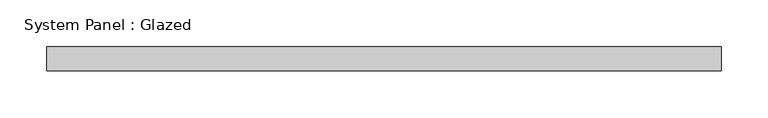
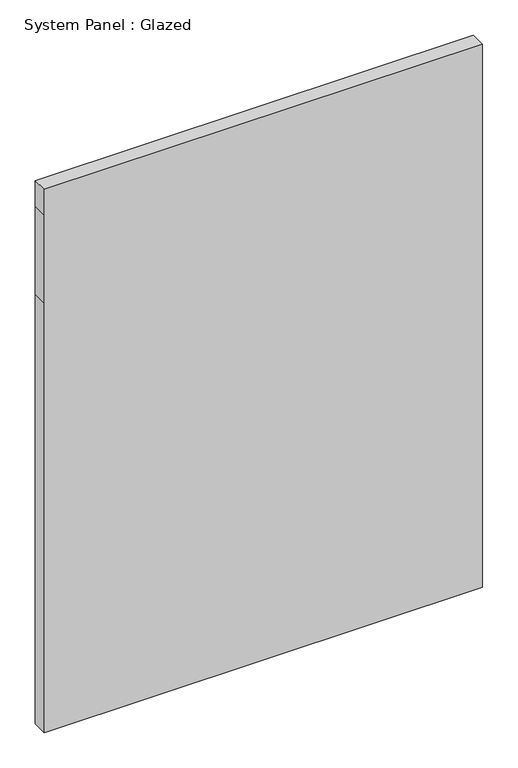
"""IFC4 building model written with IfcOpenShell, lengths in millimetres: plate geometry, System Panel : Glazed."""

from ifc_helpers import new_model, si_unit, frame, origin, place, context, project, spatial, polyline, outline, extrude, source, transform, mapped, element, save


def system_panel_glazed_be4ca357(model_context):
    return source(origin(), model_context, "Body", "SweptSolid", [
        extrude(outline(polyline([(0.0, -358.775), (0.0, 358.775), (742.6882113, 358.775), (895.0882113, 358.775), (939.5382113, 358.775), (939.5382113, -358.775), (895.0882113, -358.775), (742.6882113, -358.775), (0.0, -358.775)])), frame((0.0, 19.05, 0.0), z_axis=(0.0, 1.0, 0.0), x_axis=(0.0, 0.0, 1.0)), (0.0, 0.0, 1.0), 25.4),
    ])


if __name__ == "__main__":
    model = new_model("IFC4")
    model_context = context("Model", 3, world=origin())
    ifc_project = project(units=[si_unit("LENGTHUNIT", "METRE", prefix="MILLI")], contexts=[model_context])
    site = spatial("IfcSite", under=ifc_project)
    building = spatial("IfcBuilding", under=site)
    placement = place(None, origin())
    system_panel_glazed_shape = system_panel_glazed_be4ca357(model_context)
    element("IfcPlate", 1, ObjectType="System Panel : Glazed", at=placement, inside=building, context=model_context, shape_type="MappedRepresentation", body=[
        mapped(system_panel_glazed_shape, transform((0.0, 0.0, 0.0), x_axis=(1.0, 0.0, 0.0), y_axis=(0.0, 1.0, 0.0), z_axis=(0.0, 0.0, 1.0))),
    ])
    save(model, "model.ifc")

# Revit data of these elements
# Type "System Panel : Glazed"
#   Construction Type Id = "GSP4R"
#   Analytic Construction = "1/8 in Pilkington single glazing"
#   Visual Light Transmittance = 0.9
#   Solar Heat Gain Coefficient = 0.86
#   Heat Transfer Coefficient (U) = 1.18115 BTU/(h·ft²·°F)
#   Define Thermal Properties by = 1
# Element 1 (IfcPlate, "System Panel : Glazed")
#   Materials on its faces: "Glass"
# Materials
#   "Glass": class "Glass", colour RGB 0 128 192, transparency 0.75, Description = "Soda Lime Glass", Cost = 0
